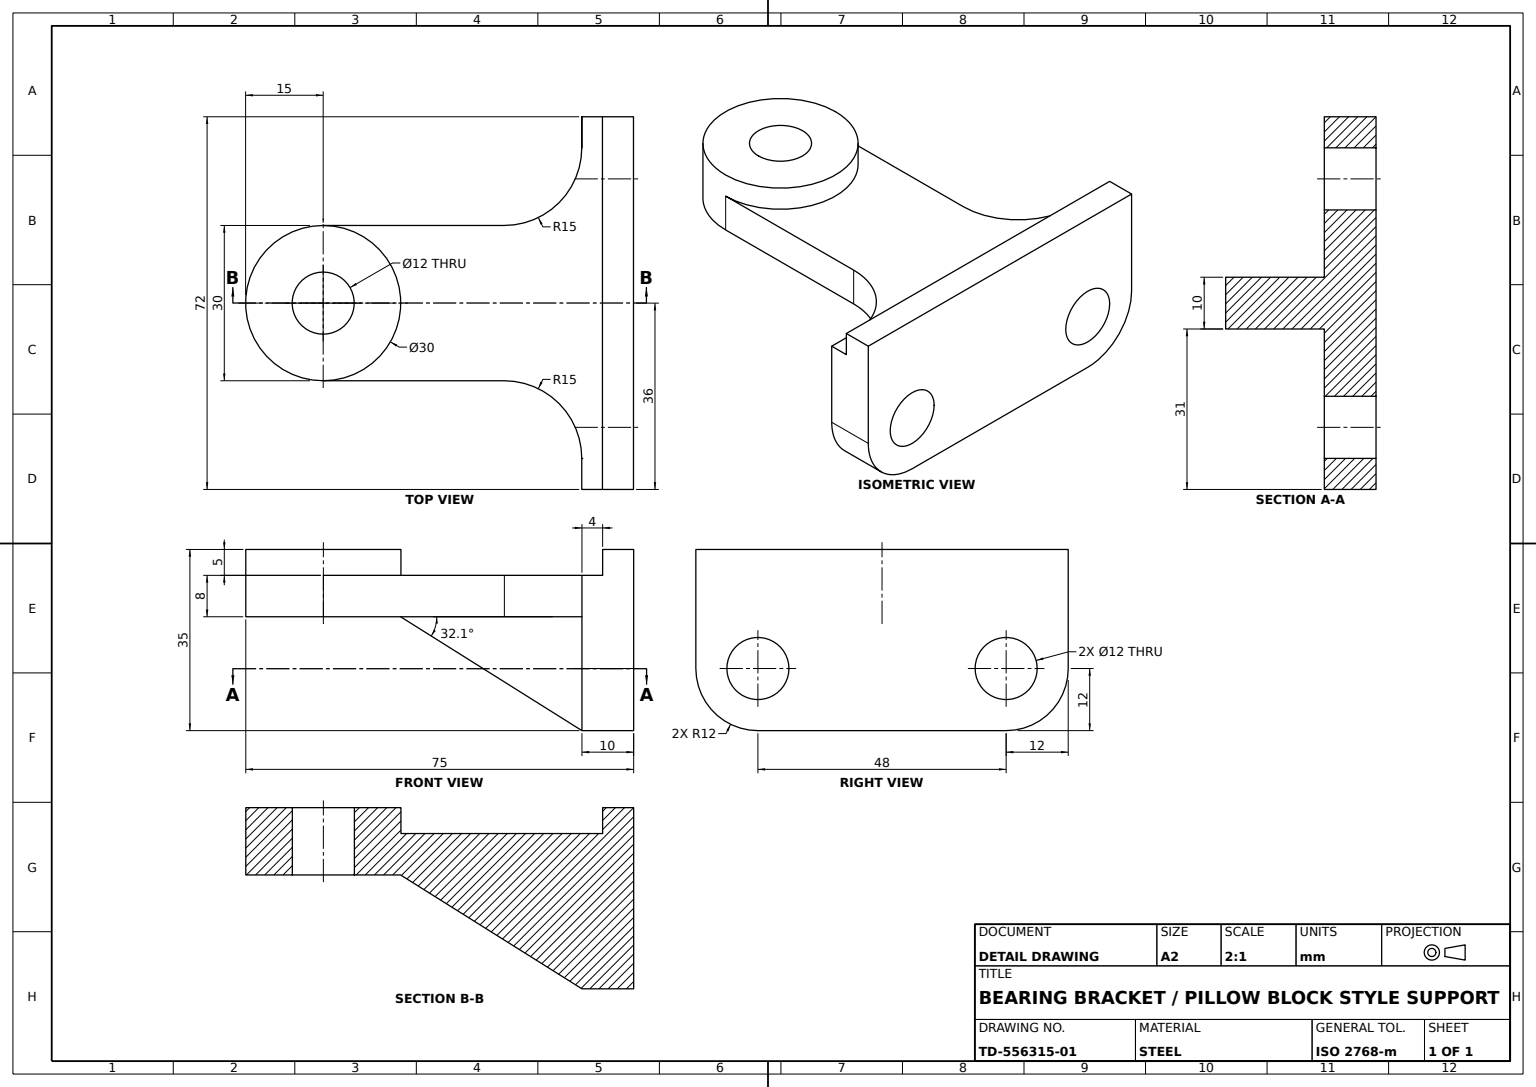
from build123d import *
from build123d.topology import SkipClean

# Parameters (mm, degrees)
BASE_PLATE_PROFILE_W   = 12
BASE_PLATE_PROFILE_H   = 23
BASE_PLATE_DEPTH       = 10
GROOVE_PROFILE_4X5_W   = 4
GROOVE_PROFILE_4X5_H   = 5
GROOVE_CUT_4X5_DEPTH   = 150
ARM_DEPTH              = 12
EYE_START              = 5
EYE_BOSS_SKETCH_30_R   = 15
EYE_BOSS_30_DEPTH      = 5
ARM_START              = -4
ARM_RELIEF_CUT_DEPTH   = 4
EYE_HOLE_SKETCH_12_R   = 6
EYE_HOLE_12_DEPTH      = 20
UPRIGHT_RIB_DEPTH      = 8
CROSS_HOLE_SKETCH_12_R = 6
CROSS_HOLE_12_DEPTH    = 20
UPRIGHT_WEB_DEPTH      = 72
WEB_TRIM_CUT_1_DEPTH   = 31
WEB_TRIM_CUT_2_DEPTH   = 31


with BuildPart() as part:
    # Base Plate Profile → Base Plate (new body)
    with BuildSketch(Plane.XY):
        Polygon((36, 0), (12, 0), (12, -23), (60, -23), (60, 0), align=None)
        with Locations((6, -11.5)):
            Rectangle(BASE_PLATE_PROFILE_W, BASE_PLATE_PROFILE_H)
        with Locations((66, -11.5)):
            Rectangle(BASE_PLATE_PROFILE_W, BASE_PLATE_PROFILE_H)
        with BuildLine():
            Line((12, -35), (60, -35))
            ThreePointArc((60, -35), (68.485281374, -31.485281374), (72, -23))
            Line((72, -23), (0, -23))
            ThreePointArc((0, -23), (3.514718626, -31.485281374), (12, -35))
        make_face()
    extrude(amount=BASE_PLATE_DEPTH)

    # Groove Profile 4x5 → Groove Cut 4x5 (cut)
    with BuildSketch(Plane(origin=(72, 0, 0), x_dir=(0, 0, -1), z_dir=(1, 0, 0))):
        with Locations((-8, -2.5)):
            Rectangle(GROOVE_PROFILE_4X5_W, GROOVE_PROFILE_4X5_H)
    extrude(amount=-GROOVE_CUT_4X5_DEPTH, mode=Mode.SUBTRACT)

    # Arm Profile → Arm (add)
    with BuildSketch(Plane(origin=(0, -5, 0), x_dir=(1, 0, 0), z_dir=(0, 1, 0))):
        with BuildLine():
            Line((21, -60), (21, -10))
            Line((21, -10), (51, -10))
            Line((51, -10), (51, -60))
            ThreePointArc((51, -60), (36, -75), (21, -60))
        make_face()
    extrude(amount=-ARM_DEPTH)

    # Eye Boss Sketch Ø30 → Eye Boss Ø30 (add)
    with SkipClean():  # the faces are left unmerged after this step: merging them gives an invalid solid
        with BuildSketch(Plane(origin=(0, -5, 0), x_dir=(1, 0, 0), z_dir=(0, 1, 0)).offset(EYE_START)):
            with Locations(Location((36, -60, 0), (0, 0, 180))):
                Circle(EYE_BOSS_SKETCH_30_R)
        extrude(amount=-EYE_BOSS_30_DEPTH)

    # Arm Relief Profile → Arm Relief Cut (cut)
    with SkipClean():  # the faces are left unmerged after this step: merging them gives an invalid solid
        with BuildSketch(Plane.XZ.offset(17).offset(ARM_START)):
            with BuildLine():
                Line((21, 10), (21, 60))
                ThreePointArc((21, 60), (36, 75), (51, 60))
                Line((51, 60), (51, 10))
                Line((51, 10), (21, 10))
            make_face()
        extrude(amount=ARM_RELIEF_CUT_DEPTH, mode=Mode.SUBTRACT)

    # Eye Hole Sketch Ø12 → Eye Hole Ø12 (cut)
    with SkipClean():  # the faces are left unmerged after this step: merging them gives an invalid solid
        with BuildSketch(Plane.XZ.offset(13)):
            with Locations((36, 60)):
                Circle(EYE_HOLE_SKETCH_12_R)
        extrude(amount=-EYE_HOLE_12_DEPTH, mode=Mode.SUBTRACT)

    # Upright Rib Profile → Upright Rib (add)
    with SkipClean():  # the faces are left unmerged after this step: merging them gives an invalid solid
        with BuildSketch(Plane.XZ.offset(13)):
            with BuildLine():
                Line((6, 10), (21, 10))
                Line((21, 10), (21, 25))
                ThreePointArc((21, 25), (16.606601718, 14.393398282), (6, 10))
            make_face()
            with BuildLine():
                Line((51, 25), (51, 10))
                Line((51, 10), (66, 10))
                ThreePointArc((66, 10), (55.393398282, 14.393398282), (51, 25))
            make_face()
        extrude(amount=-UPRIGHT_RIB_DEPTH)

    # Cross Hole Sketch Ø12 → Cross Hole Ø12 (cut)
    with SkipClean():  # the faces are left unmerged after this step: merging them gives an invalid solid
        with BuildSketch(Plane.XY.offset(10)):
            with Locations((12, -23)):
                Circle(CROSS_HOLE_SKETCH_12_R)
            with Locations((60, -23)):
                Circle(CROSS_HOLE_SKETCH_12_R)
        extrude(amount=-CROSS_HOLE_12_DEPTH, mode=Mode.SUBTRACT)

    # Upright Web Profile → Upright Web (add)
    with SkipClean():  # the faces are left unmerged after this step: merging them gives an invalid solid
        with BuildSketch(Plane.ZY):
            Polygon((10, -13), (45.07175112, -13), (10, -35), align=None)
        extrude(amount=-UPRIGHT_WEB_DEPTH)

    # Web Trim Profile 1 → Web Trim Cut 1 (cut)
    with SkipClean():  # the faces are left unmerged after this step: merging them gives an invalid solid
        with BuildSketch(Plane(origin=(72, 0, 0), x_dir=(0, 0, -1), z_dir=(1, 0, 0))):
            Polygon((-45.07175112, -13), (-10, -13), (-10, -35), align=None)
        extrude(amount=-WEB_TRIM_CUT_1_DEPTH, mode=Mode.SUBTRACT)

    # Web Trim Profile 2 → Web Trim Cut 2 (cut)
    with SkipClean():  # the faces are left unmerged after this step: merging them gives an invalid solid
        with BuildSketch(Plane.ZY):
            Polygon((10, -35), (10, -13), (45.07175112, -13), align=None)
        extrude(amount=-WEB_TRIM_CUT_2_DEPTH, mode=Mode.SUBTRACT)


solid = part.part
